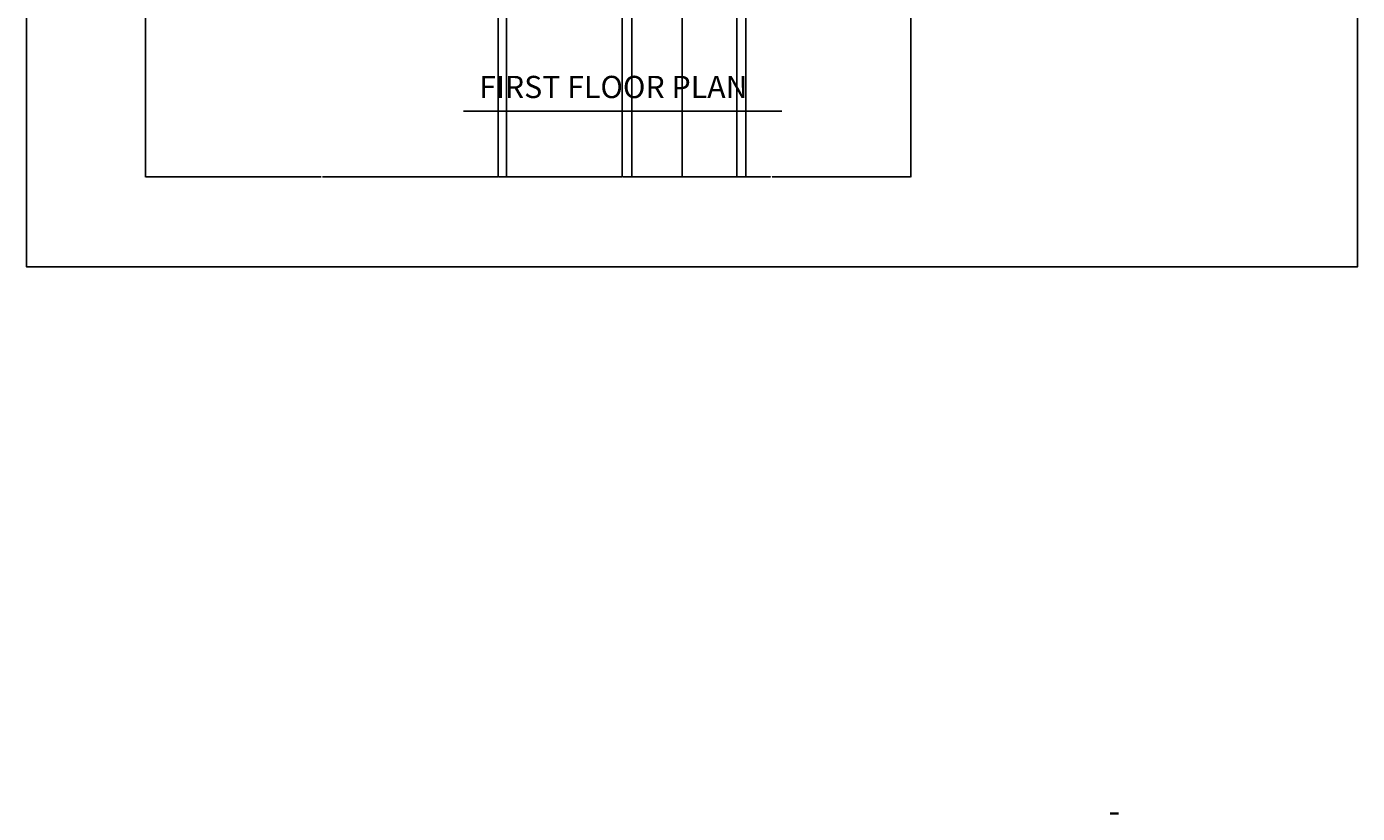
# Model space of a CAD drawing. Units: inches. Extents: x 2064 to 2782, y 1196 to 2299.
# Tile 1 of 11: x 2064 to 2782, y 1196 to 1620. Entities that reach past the tile are written whole.
import ezdxf

# ---------------------------------------------------------------- set-up
doc = ezdxf.new("R2010")
doc.units = ezdxf.units.IN
for name, color, linetype, lineweight in [('A-ANNO-DIMS', 2, 'Continuous', 18), ('A-ANNO-TTLB', 7, 'Continuous', 25), ('A-WALL', 7, 'Continuous', 35)]:
    doc.layers.add(name, color=color, linetype=linetype, lineweight=lineweight)
doc.styles.get("Standard").update_dxf_attribs({"font": 'arial.ttf'})
doc.dimstyles.get("Standard").update_dxf_attribs({"dimtxt": 0.18, "dimasz": 0.18, "dimexe": 0.18, "dimexo": 0.0625, "dimgap": 0.09, "dimtad": 0, "dimtih": 1, "dimtoh": 1, "dimdec": 4, "dimzin": 0, "dimdsep": 46, "dimtxsty": 'Standard', "dimcen": 0.09, "dimadec": 0, "dimazin": 0, "dimtfac": 1, "dimtdec": 4, "dimtofl": 0, "dimtmove": 0, "dimatfit": 3, "dimfxl": 1, "dimtolj": 1, "dimtzin": 0, "dimarcsym": 0})

# ---------------------------------------------------------------- blocks, each defined once
blk = doc.blocks.new('*D24')
at = {"layer": 'A-ANNO-DIMS', "color": 0, "lineweight": -2, "transparency": 16777216}
for p, q in [((2128.17, 1691.23), (2128.17, 1539.01)), ((2318.45, 1640.73), (2318.45, 1539.01)), ((2128.35, 1539.19), (2222.93, 1539.19)), ((2318.27, 1539.19), (2223.7, 1539.19))]:
    blk.add_line(p, q, dxfattribs=at)
at = {"layer": 'A-ANNO-DIMS', "color": 0, "transparency": 16777216}
for points in [[(2128.35, 1539.22), (2128.35, 1539.16), (2128.17, 1539.19)], [(2318.27, 1539.22), (2318.27, 1539.16), (2318.45, 1539.19)]]:
    blk.add_solid(points, dxfattribs=at)
at = {"layer": 'Defpoints', "color": 0, "transparency": 16777216}
for p in [(2128.17, 1691.29), (2318.45, 1640.79), (2318.45, 1539.19)]:
    blk.add_point(p, dxfattribs=at)
at = {"layer": 'A-ANNO-DIMS', "color": 0, "transparency": 16777216, "insert": (2223.31, 1539.19), "char_height": 0.18, "attachment_point": 5}
blk.add_mtext('\\A1;190.3', dxfattribs=at)
blk = doc.blocks.new('*D25')
at = {"layer": 'A-ANNO-DIMS', "color": 0, "lineweight": -2, "transparency": 16777216}
for p, q in [((2318.45, 1640.73), (2318.45, 1539.01)), ((2452.17, 1640.73), (2452.17, 1539.01)), ((2318.63, 1539.19), (2384.86, 1539.19)), ((2451.99, 1539.19), (2385.77, 1539.19))]:
    blk.add_line(p, q, dxfattribs=at)
at = {"layer": 'A-ANNO-DIMS', "color": 0, "transparency": 16777216}
for points in [[(2318.63, 1539.22), (2318.63, 1539.16), (2318.45, 1539.19)], [(2451.99, 1539.22), (2451.99, 1539.16), (2452.17, 1539.19)]]:
    blk.add_solid(points, dxfattribs=at)
at = {"layer": 'Defpoints', "color": 0, "transparency": 16777216}
for p in [(2318.45, 1640.79), (2452.17, 1640.79), (2452.17, 1539.19)]:
    blk.add_point(p, dxfattribs=at)
at = {"layer": 'A-ANNO-DIMS', "color": 0, "transparency": 16777216, "insert": (2385.31, 1539.19), "char_height": 0.18, "attachment_point": 5}
blk.add_mtext('\\A1;133.72', dxfattribs=at)
blk = doc.blocks.new('*D36')
at = {"layer": 'A-ANNO-DIMS', "color": 0, "lineweight": -2, "transparency": 16777216}
for p, q in [((2390.62, 2058.73), (2390.62, 1539.01)), ((2541.17, 2058.73), (2541.17, 1539.01)), ((2390.8, 1539.19), (2465.44, 1539.19)), ((2540.99, 1539.19), (2466.35, 1539.19))]:
    blk.add_line(p, q, dxfattribs=at)
at = {"layer": 'A-ANNO-DIMS', "color": 0, "transparency": 16777216}
for points in [[(2390.8, 1539.22), (2390.8, 1539.16), (2390.62, 1539.19)], [(2540.99, 1539.22), (2540.99, 1539.16), (2541.17, 1539.19)]]:
    blk.add_solid(points, dxfattribs=at)
at = {"layer": 'Defpoints', "color": 0, "transparency": 16777216}
for p in [(2390.62, 2058.79), (2541.17, 2058.79), (2541.17, 1539.19)]:
    blk.add_point(p, dxfattribs=at)
at = {"layer": 'A-ANNO-DIMS', "color": 0, "transparency": 16777216, "insert": (2465.9, 1539.19), "char_height": 0.18, "attachment_point": 5}
blk.add_mtext('\\A1;150.55', dxfattribs=at)
blk = doc.blocks.new('*D38')
at = {"layer": 'A-ANNO-DIMS', "color": 0, "lineweight": -2, "transparency": 16777216}
for p, q in [((2322.95, 1692.55), (2322.95, 1539.01)), ((2385.31, 1692.55), (2385.31, 1539.01)), ((2323.13, 1539.19), (2353.74, 1539.19)), ((2385.13, 1539.19), (2354.53, 1539.19))]:
    blk.add_line(p, q, dxfattribs=at)
at = {"layer": 'A-ANNO-DIMS', "color": 0, "transparency": 16777216}
for points in [[(2323.13, 1539.22), (2323.13, 1539.16), (2322.95, 1539.19)], [(2385.13, 1539.22), (2385.13, 1539.16), (2385.31, 1539.19)]]:
    blk.add_solid(points, dxfattribs=at)
at = {"layer": 'Defpoints', "color": 0, "transparency": 16777216}
for p in [(2322.95, 1692.61), (2385.31, 1692.61), (2385.31, 1539.19)]:
    blk.add_point(p, dxfattribs=at)
at = {"layer": 'A-ANNO-DIMS', "color": 0, "transparency": 16777216, "insert": (2354.13, 1539.19), "char_height": 0.18, "attachment_point": 5}
blk.add_mtext('\\A1;62.36', dxfattribs=at)
blk = doc.blocks.new('*D41')
at = {"layer": 'A-ANNO-DIMS', "color": 0, "lineweight": -2, "transparency": 16777216}
for p, q in [((2417.67, 2229.73), (2417.67, 1539.01)), ((2447.29, 2229.73), (2447.29, 1539.01)), ((2417.85, 1539.19), (2432.08, 1539.19)), ((2447.11, 1539.19), (2432.87, 1539.19))]:
    blk.add_line(p, q, dxfattribs=at)
at = {"layer": 'A-ANNO-DIMS', "color": 0, "transparency": 16777216}
for points in [[(2417.85, 1539.22), (2417.85, 1539.16), (2417.67, 1539.19)], [(2447.11, 1539.22), (2447.11, 1539.16), (2447.29, 1539.19)]]:
    blk.add_solid(points, dxfattribs=at)
at = {"layer": 'Defpoints', "color": 0, "transparency": 16777216}
for p in [(2417.67, 2229.79), (2447.29, 2229.79), (2447.29, 1539.19)]:
    blk.add_point(p, dxfattribs=at)
at = {"layer": 'A-ANNO-DIMS', "color": 0, "transparency": 16777216, "insert": (2432.48, 1539.19), "char_height": 0.18, "attachment_point": 5}
blk.add_mtext('\\A1;29.62', dxfattribs=at)

msp = doc.modelspace()

# ---------------------------------------------------------------- linework, layer by layer
at = {"layer": 'A-ANNO-TTLB'}
msp.add_line((2299.8295, 1574.6896), (2471.6072, 1574.6896), dxfattribs=at)
msp.add_lwpolyline([(2063.9994, 2298.574), (2782.0941, 2298.574), (2782.0941, 1490.6238), (2063.9994, 1490.6238)], close=True, dxfattribs=at)
at = {"layer": 'A-WALL'}
msp.add_line((2653.1691, 1195.6864), (2648.6691, 1195.6864), dxfattribs=at)

# ---------------------------------------------------------------- texts
at = {"layer": 'A-ANNO-TTLB', "insert": (2308.2423, 1593.7667), "char_height": 12, "attachment_point": 1}
msp.add_mtext_dynamic_manual_height_columns('FIRST FLOOR PLAN', width=467.865449, gutter_width=12.5, heights=[0], dxfattribs=at)

# ---------------------------------------------------------------- dimensions: what is measured, and where the dimension line sits
at = {"layer": 'A-ANNO-DIMS'}
for base, p1, p2, override, picture, middle in [((2447.2886, 1539.1896), (2417.6691, 2229.7917), (2447.2886, 2229.7917), {"dimdec": 2, "dimlfac": 1, "dimrnd": 0, "dimzin": 0, "dimdsep": 46, "dimlunit": 2}, '*D41', (2432.4788, 1539.1896)), ((2541.1691, 1539.1896), (2390.6222, 2058.7917), (2541.1691, 2058.7917), {"dimdec": 2, "dimlfac": 1, "dimrnd": 0, "dimzin": 0, "dimdsep": 46, "dimlunit": 2}, '*D36', (2465.8957, 1539.1896)), ((2318.4532, 1539.1896), (2128.1691, 1691.2917), (2318.4532, 1640.7917), {"dimdec": 1, "dimlfac": 1, "dimrnd": 0, "dimzin": 0, "dimdsep": 46, "dimlunit": 2}, '*D24', (2223.3112, 1539.1896)), ((2385.3111, 1539.1896), (2322.9532, 1692.6099), (2385.3111, 1692.6099), {"dimdec": 2, "dimlfac": 1, "dimrnd": 0, "dimzin": 0, "dimdsep": 46, "dimlunit": 2}, '*D38', (2354.1322, 1539.1896)), ((2452.1691, 1539.1896), (2318.4532, 1640.7917), (2452.1691, 1640.7917), {"dimdec": 2, "dimlfac": 1, "dimrnd": 0, "dimzin": 0, "dimdsep": 46, "dimlunit": 2}, '*D25', (2385.3112, 1539.1896))]:
    dim = msp.add_linear_dim(base=base, p1=p1, p2=p2, dimstyle='Standard', override=override, dxfattribs=at)
    dim.commit()
    dim.dimension.update_dxf_attribs({"geometry": picture, "text_midpoint": middle})

doc.saveas('drawing.dxf')
